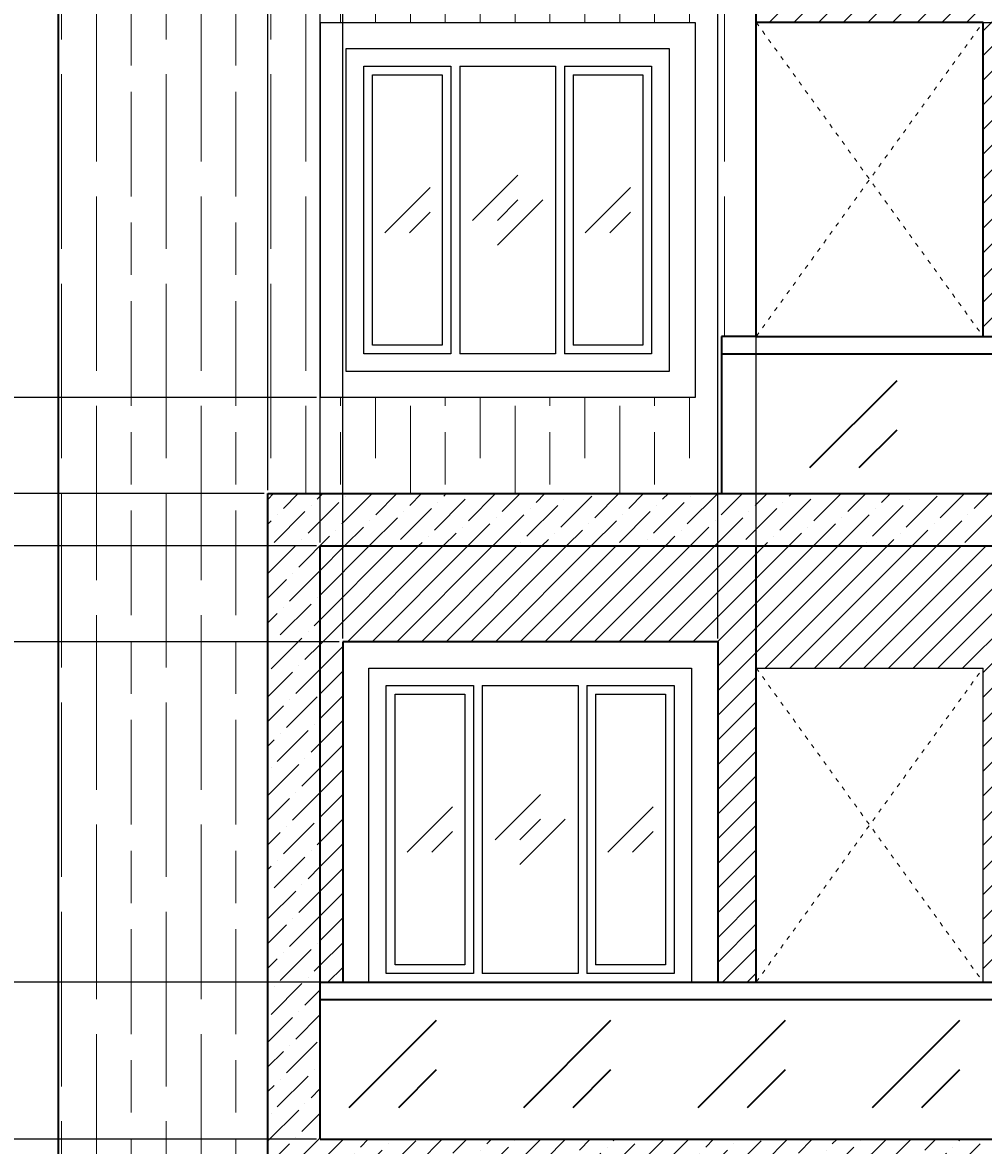
# Model space of a CAD drawing. Units: millimetres. Extents: x -692 to 9639, y -141 to 10345.
# Tile 13 of 19: x 3088 to 5843, y 4981 to 8199. Entities that reach past the tile are written whole.
import ezdxf

# ---------------------------------------------------------------- set-up
doc = ezdxf.new("R2010")
doc.units = ezdxf.units.MM
doc.header["$MEASUREMENT"] = 0
doc.linetypes.add('ACAD_ISO03W100', pattern=[30, 12, -18])
for name, color, linetype, lineweight in [('A-ANNO-DIMS', 2, 'Continuous', 18), ('A-DOOR', 3, 'Continuous', 25), ('A-DOOR-SWNG', 3, 'ACAD_ISO03W100', 18), ('A-ELEV', 7, 'Continuous', 35), ('A-ELEV-PATT', 8, 'Continuous', 13), ('A-GLAZ', 4, 'Continuous', 25)]:
    doc.layers.add(name, color=color, linetype=linetype, lineweight=lineweight)
doc.styles.get("Standard").update_dxf_attribs({"font": 'arial.ttf'})
doc.dimstyles.get("Standard").update_dxf_attribs({"dimtxt": 25, "dimasz": 20, "dimexe": 0.18, "dimexo": 10, "dimgap": 10, "dimtad": 0, "dimtih": 1, "dimtoh": 1, "dimdec": 0, "dimzin": 0, "dimdsep": 46, "dimtxsty": 'Standard', "dimcen": 10, "dimadec": 0, "dimazin": 0, "dimtfac": 1, "dimtdec": 0, "dimtofl": 0, "dimtmove": 0, "dimatfit": 3, "dimfxl": 1, "dimtolj": 1, "dimtzin": 0, "dimarcsym": 0})

# ---------------------------------------------------------------- blocks, each defined once
blk = doc.blocks.new('WIN-1075')
for p, q in [((0, 1075), (1075, 1075)), ((0, 1075), (0, 0)), ((1075, 1075), (1075, 0)), ((75, 1000), (1000, 1000)), ((75, 75), (75, 1000)), ((1000, 1000), (1000, 75)), ((125, 950), (375, 950)), ((125, 125), (125, 950)), ((375, 950), (375, 125)), ((400, 950), (400, 125)), ((400, 950), (675, 950)), ((675, 950), (675, 125)), ((700, 950), (700, 125)), ((700, 950), (950, 950)), ((950, 950), (950, 125)), ((150, 150), (150, 925)), ((150, 925), (350, 925)), ((350, 925), (350, 150)), ((725, 925), (725, 150)), ((725, 925), (925, 925)), ((925, 925), (925, 150)), ((567.1, 637.9), (437.1, 507.9)), ((315, 602.5), (185, 472.5)), ((890, 602.5), (760, 472.5)), ((637.9, 567.1), (507.9, 437.1)), ((567.1, 567.1), (507.9, 507.9)), ((315, 531.8), (255.7, 472.5)), ((890, 531.8), (830.7, 472.5)), ((350, 150), (150, 150)), ((925, 150), (725, 150)), ((375, 125), (125, 125)), ((675, 125), (400, 125)), ((950, 125), (700, 125)), ((1000, 75), (75, 75)), ((1075, 0), (0, 0))]:
    blk.add_line(p, q)
blk = doc.blocks.new('*D7')
at = {"layer": 'A-ANNO-DIMS', "color": 0, "lineweight": -2, "transparency": 16777216}
for p, q in [((8481.5, 9848.8), (-649.1, 9848.8)), ((-648.9, 9828.8), (-648.9, 5124.9)), ((-648.9, 375.6), (-648.9, 5079.4)), ((2463.7, 355.6), (-649.1, 355.6))]:
    blk.add_line(p, q, dxfattribs=at)
at = {"layer": 'A-ANNO-DIMS', "color": 0, "lineweight": -3, "transparency": 16777216}
for points in [[(-652.2, 9828.8), (-645.6, 9828.8), (-648.9, 9848.8)], [(-652.2, 375.6), (-645.6, 375.6), (-648.9, 355.6)]]:
    blk.add_solid(points, dxfattribs=at)
at = {"layer": 'Defpoints', "color": 0, "lineweight": -3, "transparency": 16777216}
for p in [(-648.9, 9848.8), (8491.5, 9848.8), (2473.7, 355.6)]:
    blk.add_point(p, dxfattribs=at)
at = {"layer": 'A-ANNO-DIMS', "color": 0, "transparency": 16777216, "insert": (-648.9, 5102.2), "char_height": 25, "attachment_point": 5}
blk.add_mtext('\\A1;9493', dxfattribs=at)
blk = doc.blocks.new('*D52')
at = {"layer": 'A-ANNO-DIMS', "color": 0, "lineweight": -2, "transparency": 16777216}
for p, q in [((3791.5, 6858.8), (3791.5, 10329)), ((3811.5, 10328.8), (3830.1, 10328.8)), ((3921.5, 10328.8), (3902.9, 10328.8)), ((3941.5, 6708.8), (3941.5, 10329))]:
    blk.add_line(p, q, dxfattribs=at)
at = {"layer": 'A-ANNO-DIMS', "color": 0, "lineweight": -3, "transparency": 16777216}
for points in [[(3811.5, 10332.1), (3811.5, 10325.4), (3791.5, 10328.8)], [(3921.5, 10332.1), (3921.5, 10325.4), (3941.5, 10328.8)]]:
    blk.add_solid(points, dxfattribs=at)
at = {"layer": 'Defpoints', "color": 0, "lineweight": -3, "transparency": 16777216}
for p in [(3941.5, 10328.8), (3791.5, 6848.8), (3941.5, 6698.8)]:
    blk.add_point(p, dxfattribs=at)
at = {"layer": 'A-ANNO-DIMS', "color": 0, "transparency": 16777216, "insert": (3866.5, 10328.8), "char_height": 25, "attachment_point": 5}
blk.add_mtext('\\A1;150', dxfattribs=at)
blk = doc.blocks.new('*D53')
at = {"layer": 'A-ANNO-DIMS', "color": 0, "lineweight": -2, "transparency": 16777216}
for p, q in [((3941.5, 6708.8), (3941.5, 10329)), ((3961.5, 10328.8), (3986.3, 10328.8)), ((4006.3, 6433.8), (4006.3, 10329)), ((4006.3, 10328.8), (4026.3, 10328.8))]:
    blk.add_line(p, q, dxfattribs=at)
at = {"layer": 'A-ANNO-DIMS', "color": 0, "lineweight": -3, "transparency": 16777216}
for points in [[(3961.5, 10332.1), (3961.5, 10325.4), (3941.5, 10328.8)], [(3986.3, 10332.1), (3986.3, 10325.4), (4006.3, 10328.8)]]:
    blk.add_solid(points, dxfattribs=at)
at = {"layer": 'Defpoints', "color": 0, "lineweight": -3, "transparency": 16777216}
for p in [(4006.3, 10328.8), (3941.5, 6698.8), (4006.3, 6423.8)]:
    blk.add_point(p, dxfattribs=at)
at = {"layer": 'A-ANNO-DIMS', "color": 0, "transparency": 16777216, "insert": (4076.1, 10328.8), "char_height": 25, "attachment_point": 5}
blk.add_mtext('\\A1;64.71', dxfattribs=at)
blk = doc.blocks.new('*D54')
at = {"layer": 'A-ANNO-DIMS', "color": 0, "lineweight": -2, "transparency": 16777216}
for p, q in [((4006.3, 6433.8), (4006.3, 10329)), ((4026.3, 10328.8), (4497.5, 10328.8)), ((5061.3, 10328.8), (4590, 10328.8)), ((5081.3, 6433.8), (5081.3, 10329))]:
    blk.add_line(p, q, dxfattribs=at)
at = {"layer": 'A-ANNO-DIMS', "color": 0, "lineweight": -3, "transparency": 16777216}
for points in [[(4026.3, 10332.1), (4026.3, 10325.4), (4006.3, 10328.8)], [(5061.3, 10332.1), (5061.3, 10325.4), (5081.3, 10328.8)]]:
    blk.add_solid(points, dxfattribs=at)
at = {"layer": 'Defpoints', "color": 0, "lineweight": -3, "transparency": 16777216}
for p in [(5081.3, 10328.8), (4006.3, 6423.8), (5081.3, 6423.8)]:
    blk.add_point(p, dxfattribs=at)
at = {"layer": 'A-ANNO-DIMS', "color": 0, "transparency": 16777216, "insert": (4543.8, 10328.8), "char_height": 25, "attachment_point": 5}
blk.add_mtext('\\A1;1075', dxfattribs=at)
blk = doc.blocks.new('*D55')
at = {"layer": 'A-ANNO-DIMS', "color": 0, "lineweight": -2, "transparency": 16777216}
for p, q in [((5081.3, 6433.8), (5081.3, 10329)), ((5101.3, 10328.8), (5171.5, 10328.8)), ((5191.5, 6358.8), (5191.5, 10329)), ((5191.5, 10328.8), (5211.5, 10328.8))]:
    blk.add_line(p, q, dxfattribs=at)
at = {"layer": 'A-ANNO-DIMS', "color": 0, "lineweight": -3, "transparency": 16777216}
for points in [[(5101.3, 10332.1), (5101.3, 10325.4), (5081.3, 10328.8)], [(5171.5, 10332.1), (5171.5, 10325.4), (5191.5, 10328.8)]]:
    blk.add_solid(points, dxfattribs=at)
at = {"layer": 'Defpoints', "color": 0, "lineweight": -3, "transparency": 16777216}
for p in [(5191.5, 10328.8), (5081.3, 6423.8), (5191.5, 6348.8)]:
    blk.add_point(p, dxfattribs=at)
at = {"layer": 'A-ANNO-DIMS', "color": 0, "transparency": 16777216, "insert": (5272.3, 10328.8), "char_height": 25, "attachment_point": 5}
blk.add_mtext('\\A1;110.29', dxfattribs=at)
blk = doc.blocks.new('*D56')
at = {"layer": 'A-ANNO-DIMS', "color": 0, "lineweight": -2, "transparency": 16777216}
for p, q in [((5191.5, 6358.8), (5191.5, 10329)), ((5211.5, 10328.8), (5981.1, 10328.8)), ((6871.7, 10328.8), (6102.2, 10328.8)), ((6891.7, 6708.8), (6891.7, 10329))]:
    blk.add_line(p, q, dxfattribs=at)
at = {"layer": 'A-ANNO-DIMS', "color": 0, "lineweight": -3, "transparency": 16777216}
for points in [[(5211.5, 10332.1), (5211.5, 10325.4), (5191.5, 10328.8)], [(6871.7, 10332.1), (6871.7, 10325.4), (6891.7, 10328.8)]]:
    blk.add_solid(points, dxfattribs=at)
at = {"layer": 'Defpoints', "color": 0, "lineweight": -3, "transparency": 16777216}
for p in [(6891.7, 10328.8), (6891.7, 6698.8), (5191.5, 6348.8)]:
    blk.add_point(p, dxfattribs=at)
at = {"layer": 'A-ANNO-DIMS', "color": 0, "transparency": 16777216, "insert": (6041.6, 10328.8), "char_height": 25, "attachment_point": 5}
blk.add_mtext('\\A1;1700.2', dxfattribs=at)
blk = doc.blocks.new('*D63')
at = {"layer": 'A-ANNO-DIMS', "color": 0, "lineweight": -2, "transparency": 16777216}
for p, q in [((3931.5, 4998.8), (-649.1, 4998.8)), ((-648.9, 4978.8), (-648.9, 4946.5)), ((-648.9, 4868.8), (-648.9, 4901)), ((3781.5, 4848.8), (-649.1, 4848.8))]:
    blk.add_line(p, q, dxfattribs=at)
at = {"layer": 'A-ANNO-DIMS', "color": 0, "lineweight": -3, "transparency": 16777216}
for points in [[(-652.2, 4978.8), (-645.6, 4978.8), (-648.9, 4998.8)], [(-652.2, 4868.8), (-645.6, 4868.8), (-648.9, 4848.8)]]:
    blk.add_solid(points, dxfattribs=at)
at = {"layer": 'Defpoints', "color": 0, "lineweight": -3, "transparency": 16777216}
for p in [(-648.9, 4998.8), (3941.5, 4998.8), (3791.5, 4848.8)]:
    blk.add_point(p, dxfattribs=at)
at = {"layer": 'A-ANNO-DIMS', "color": 0, "transparency": 16777216, "insert": (-648.9, 4923.8), "char_height": 25, "attachment_point": 5}
blk.add_mtext('\\A1;150', dxfattribs=at)
blk = doc.blocks.new('*D64')
at = {"layer": 'A-ANNO-DIMS', "color": 0, "lineweight": -2, "transparency": 16777216}
for p, q in [((3996.3, 5448.8), (-649.1, 5448.8)), ((-648.9, 5428.8), (-648.9, 5246.5)), ((-648.9, 5018.8), (-648.9, 5201)), ((3931.5, 4998.8), (-649.1, 4998.8))]:
    blk.add_line(p, q, dxfattribs=at)
at = {"layer": 'A-ANNO-DIMS', "color": 0, "lineweight": -3, "transparency": 16777216}
for points in [[(-652.2, 5428.8), (-645.6, 5428.8), (-648.9, 5448.8)], [(-652.2, 5018.8), (-645.6, 5018.8), (-648.9, 4998.8)]]:
    blk.add_solid(points, dxfattribs=at)
at = {"layer": 'Defpoints', "color": 0, "lineweight": -3, "transparency": 16777216}
for p in [(-648.9, 5448.8), (4006.3, 5448.8), (3941.5, 4998.8)]:
    blk.add_point(p, dxfattribs=at)
at = {"layer": 'A-ANNO-DIMS', "color": 0, "transparency": 16777216, "insert": (-648.9, 5223.8), "char_height": 25, "attachment_point": 5}
blk.add_mtext('\\A1;450', dxfattribs=at)
blk = doc.blocks.new('*D65')
at = {"layer": 'A-ANNO-DIMS', "color": 0, "lineweight": -2, "transparency": 16777216}
for p, q in [((3996.3, 6423.8), (-649.1, 6423.8)), ((-648.9, 6403.8), (-648.9, 5959)), ((-648.9, 5468.8), (-648.9, 5913.5)), ((3996.3, 5448.8), (-649.1, 5448.8))]:
    blk.add_line(p, q, dxfattribs=at)
at = {"layer": 'A-ANNO-DIMS', "color": 0, "lineweight": -3, "transparency": 16777216}
for points in [[(-652.2, 6403.8), (-645.6, 6403.8), (-648.9, 6423.8)], [(-652.2, 5468.8), (-645.6, 5468.8), (-648.9, 5448.8)]]:
    blk.add_solid(points, dxfattribs=at)
at = {"layer": 'Defpoints', "color": 0, "lineweight": -3, "transparency": 16777216}
for p in [(-648.9, 6423.8), (4006.3, 6423.8), (4006.3, 5448.8)]:
    blk.add_point(p, dxfattribs=at)
at = {"layer": 'A-ANNO-DIMS', "color": 0, "transparency": 16777216, "insert": (-648.9, 5936.3), "char_height": 25, "attachment_point": 5}
blk.add_mtext('\\A1;975', dxfattribs=at)
blk = doc.blocks.new('*D66')
at = {"layer": 'A-ANNO-DIMS', "color": 0, "lineweight": -2, "transparency": 16777216}
for p, q in [((3931.5, 6698.8), (-649.1, 6698.8)), ((-648.9, 6678.8), (-648.9, 6584)), ((-648.9, 6443.8), (-648.9, 6538.5)), ((3996.3, 6423.8), (-649.1, 6423.8))]:
    blk.add_line(p, q, dxfattribs=at)
at = {"layer": 'A-ANNO-DIMS', "color": 0, "lineweight": -3, "transparency": 16777216}
for points in [[(-652.2, 6678.8), (-645.6, 6678.8), (-648.9, 6698.8)], [(-652.2, 6443.8), (-645.6, 6443.8), (-648.9, 6423.8)]]:
    blk.add_solid(points, dxfattribs=at)
at = {"layer": 'Defpoints', "color": 0, "lineweight": -3, "transparency": 16777216}
for p in [(-648.9, 6698.8), (3941.5, 6698.8), (4006.3, 6423.8)]:
    blk.add_point(p, dxfattribs=at)
at = {"layer": 'A-ANNO-DIMS', "color": 0, "transparency": 16777216, "insert": (-648.9, 6561.3), "char_height": 25, "attachment_point": 5}
blk.add_mtext('\\A1;275', dxfattribs=at)
blk = doc.blocks.new('*D67')
at = {"layer": 'A-ANNO-DIMS', "color": 0, "lineweight": -2, "transparency": 16777216}
for p, q in [((3781.5, 6848.8), (-649.1, 6848.8)), ((-648.9, 6828.8), (-648.9, 6796.5)), ((-648.9, 6718.8), (-648.9, 6751)), ((3931.5, 6698.8), (-649.1, 6698.8))]:
    blk.add_line(p, q, dxfattribs=at)
at = {"layer": 'A-ANNO-DIMS', "color": 0, "lineweight": -3, "transparency": 16777216}
for points in [[(-652.2, 6828.8), (-645.6, 6828.8), (-648.9, 6848.8)], [(-652.2, 6718.8), (-645.6, 6718.8), (-648.9, 6698.8)]]:
    blk.add_solid(points, dxfattribs=at)
at = {"layer": 'Defpoints', "color": 0, "lineweight": -3, "transparency": 16777216}
for p in [(-648.9, 6848.8), (3791.5, 6848.8), (3941.5, 6698.8)]:
    blk.add_point(p, dxfattribs=at)
at = {"layer": 'A-ANNO-DIMS', "color": 0, "transparency": 16777216, "insert": (-648.9, 6773.8), "char_height": 25, "attachment_point": 5}
blk.add_mtext('\\A1;150', dxfattribs=at)
blk = doc.blocks.new('*D68')
at = {"layer": 'A-ANNO-DIMS', "color": 0, "lineweight": -2, "transparency": 16777216}
for p, q in [((3931.5, 7123.8), (-649.1, 7123.8)), ((-648.9, 7103.8), (-648.9, 7009)), ((-648.9, 6868.8), (-648.9, 6963.5)), ((3781.5, 6848.8), (-649.1, 6848.8))]:
    blk.add_line(p, q, dxfattribs=at)
at = {"layer": 'A-ANNO-DIMS', "color": 0, "lineweight": -3, "transparency": 16777216}
for points in [[(-652.2, 7103.8), (-645.6, 7103.8), (-648.9, 7123.8)], [(-652.2, 6868.8), (-645.6, 6868.8), (-648.9, 6848.8)]]:
    blk.add_solid(points, dxfattribs=at)
at = {"layer": 'Defpoints', "color": 0, "lineweight": -3, "transparency": 16777216}
for p in [(-648.9, 7123.8), (3941.5, 7123.8), (3791.5, 6848.8)]:
    blk.add_point(p, dxfattribs=at)
at = {"layer": 'A-ANNO-DIMS', "color": 0, "transparency": 16777216, "insert": (-648.9, 6986.3), "char_height": 25, "attachment_point": 5}
blk.add_mtext('\\A1;275', dxfattribs=at)
blk = doc.blocks.new('*D76')
at = {"layer": 'A-ANNO-DIMS', "color": 0, "lineweight": -2, "transparency": 16777216}
for p, q in [((5101.5, 7298.8), (9553.9, 7298.8)), ((9553.7, 7278.8), (9553.7, 7096.5)), ((9553.7, 6868.8), (9553.7, 7051)), ((5101.5, 6848.8), (9553.9, 6848.8))]:
    blk.add_line(p, q, dxfattribs=at)
at = {"layer": 'A-ANNO-DIMS', "color": 0, "lineweight": -3, "transparency": 16777216}
for points in [[(9550.4, 7278.8), (9557.1, 7278.8), (9553.7, 7298.8)], [(9550.4, 6868.8), (9557.1, 6868.8), (9553.7, 6848.8)]]:
    blk.add_solid(points, dxfattribs=at)
at = {"layer": 'Defpoints', "color": 0, "lineweight": -3, "transparency": 16777216}
for p in [(5091.5, 7298.8), (9553.7, 7298.8), (5091.5, 6848.8)]:
    blk.add_point(p, dxfattribs=at)
at = {"layer": 'A-ANNO-DIMS', "color": 0, "transparency": 16777216, "insert": (9553.7, 7073.8), "char_height": 25, "attachment_point": 5}
blk.add_mtext('\\A1;450', dxfattribs=at)
blk = doc.blocks.new('*D77')
at = {"layer": 'A-ANNO-DIMS', "color": 0, "lineweight": -2, "transparency": 16777216}
for p, q in [((5201.5, 8198.8), (9553.9, 8198.8)), ((9553.7, 8178.8), (9553.7, 7771.8)), ((9553.7, 7319.3), (9553.7, 7726.3)), ((5201.5, 7299.3), (9553.9, 7299.3))]:
    blk.add_line(p, q, dxfattribs=at)
at = {"layer": 'A-ANNO-DIMS', "color": 0, "lineweight": -3, "transparency": 16777216}
for points in [[(9550.4, 8178.8), (9557.1, 8178.8), (9553.7, 8198.8)], [(9550.4, 7319.3), (9557.1, 7319.3), (9553.7, 7299.3)]]:
    blk.add_solid(points, dxfattribs=at)
at = {"layer": 'Defpoints', "color": 0, "lineweight": -3, "transparency": 16777216}
for p in [(5191.5, 8198.8), (9553.7, 8198.8), (5191.5, 7299.3)]:
    blk.add_point(p, dxfattribs=at)
at = {"layer": 'A-ANNO-DIMS', "color": 0, "transparency": 16777216, "insert": (9553.7, 7749), "char_height": 25, "attachment_point": 5}
blk.add_mtext('\\A1;899.5', dxfattribs=at)

msp = doc.modelspace()

# ---------------------------------------------------------------- hatches: boundary and pattern name
at = {"layer": 'A-ELEV-PATT'}
h = msp.add_hatch(dxfattribs=at)
h.set_pattern_fill('GOST_WOOD', color=256, scale=50)
h.set_pattern_definition([(90, (0, 0), (300, -2e-14), [500, -100]), (90, (100, -100), (300, -2e-14), [300, -75, 150, -75]), (90, (200, -250), (300, -2e-14), [500, -100])])
edge = h.paths.add_edge_path()
edge.add_line((5191.547, 8748.772), (3791.547, 8748.772))
edge.add_line((3791.547, 8748.772), (3791.547, 8848.772))
edge.add_line((3791.547, 8848.772), (5191.547, 8848.772))
edge.add_line((5191.547, 8848.772), (5191.547, 9348.772))
edge.add_line((5191.547, 9348.772), (4755.992, 9348.772))
edge.add_line((4755.992, 9348.772), (4755.854, 9348.465))
edge.add_line((4755.854, 9348.465), (4755.734, 9348.772))
edge.add_line((4755.734, 9348.772), (4053.129, 9348.772))
edge.add_line((4053.129, 9348.772), (4052.99, 9348.465))
edge.add_line((4052.99, 9348.465), (4052.871, 9348.772))
edge.add_line((4052.871, 9348.772), (3701.731, 9348.772))
edge.add_line((3701.731, 9348.772), (3701.593, 9348.465))
edge.add_line((3701.593, 9348.465), (3701.474, 9348.772))
edge.add_line((3701.474, 9348.772), (3368.199, 9348.772))
edge.add_line((3368.199, 9348.772), (3368.061, 9348.465))
edge.add_line((3368.061, 9348.465), (3367.942, 9348.772))
edge.add_line((3367.942, 9348.772), (3191.547, 9348.772))
edge.add_line((3191.547, 9348.772), (3191.547, 3210.058))
edge.add_spline(control_points=[(3191.547, 3210.058), (3198.467, 3207.5), (3283.859, 3166.656), (3324.053, 2995.08), (3234.02, 2920.058), (3220.783, 2911.684)], knot_values=[13649.89756952, 13649.89756952, 13649.89756952, 13649.89756952, 13672.14990348, 13935.42377748, 13974.4426778, 13974.4426778, 13974.4426778, 13974.4426778], degree=3, periodic=0)
edge.add_spline(control_points=[(3220.783, 2911.684), (3225.148, 2890.107), (3226.864, 2868.931), (3226.144, 2848.27)], knot_values=[8828.69997321, 8828.69997321, 8828.69997321, 8828.69997321, 8890.6429847, 8890.6429847, 8890.6429847, 8890.6429847], degree=3, periodic=0)
edge.add_line((3226.144, 2848.27), (5191.547, 2848.27))
edge.add_line((5191.547, 2848.27), (5191.547, 3048.27))
edge.add_line((5191.547, 3048.27), (5041.547, 3048.27))
edge.add_line((5041.547, 3048.27), (5041.547, 3148.27))
edge.add_line((5041.547, 3148.27), (5091.547, 3148.27))
edge.add_line((5091.547, 3148.27), (5091.547, 3598.27))
edge.add_line((5091.547, 3598.27), (5191.547, 3598.27))
edge.add_line((5191.547, 3598.27), (5191.547, 4848.772))
edge.add_line((5191.547, 4848.772), (3791.547, 4848.772))
edge.add_line((3791.547, 4848.772), (3791.547, 6848.772))
edge.add_line((3791.547, 6848.772), (5091.547, 6848.772))
edge.add_line((5091.547, 6848.772), (5091.547, 7298.772))
edge.add_line((5091.547, 7298.772), (5191.547, 7298.772))
edge.add_line((5191.547, 7298.772), (5191.547, 8748.772))
h.paths.add_polyline_path([(5016.547, 8198.772), (5016.547, 7123.772), (3941.547, 7123.772), (3941.547, 8198.772)], flags=16)
h.paths.add_polyline_path([(4941.547, 8123.772), (4941.547, 7198.772), (4016.547, 7198.772), (4016.547, 8123.772)], flags=0)
h.paths.add_polyline_path([(4616.547, 8073.772), (4616.547, 7248.772), (4341.547, 7248.772), (4341.547, 8073.772)], flags=0)
h.paths.add_polyline_path([(4641.547, 8073.772), (4891.547, 8073.772), (4891.547, 7248.772), (4641.547, 7248.772)], flags=0)
h.paths.add_polyline_path([(4666.547, 8048.772), (4866.547, 8048.772), (4866.547, 7273.772), (4666.547, 7273.772)], flags=0)
h.paths.add_polyline_path([(4316.547, 8073.772), (4316.547, 7248.772), (4066.547, 7248.772), (4066.547, 8073.772)], flags=0)
h.paths.add_polyline_path([(4291.547, 8048.772), (4291.547, 7273.772), (4091.547, 7273.772), (4091.547, 8048.772)], flags=0)
h.paths.add_polyline_path([(5016.547, 4497.772), (5016.547, 3422.772), (3941.547, 3422.772), (3941.547, 4497.772)], flags=16)
h.paths.add_polyline_path([(4941.547, 4422.772), (4941.547, 3497.772), (4016.547, 3497.772), (4016.547, 4422.772)], flags=0)
h.paths.add_polyline_path([(4616.547, 4372.772), (4616.547, 3547.772), (4341.547, 3547.772), (4341.547, 4372.772)], flags=0)
h.paths.add_polyline_path([(4641.547, 4372.772), (4891.547, 4372.772), (4891.547, 3547.772), (4641.547, 3547.772)], flags=0)
h.paths.add_polyline_path([(4316.547, 4372.772), (4316.547, 3547.772), (4066.547, 3547.772), (4066.547, 4372.772)], flags=0)
h.paths.add_polyline_path([(4666.547, 4347.772), (4866.547, 4347.772), (4866.547, 3572.772), (4666.547, 3572.772)], flags=0)
h.paths.add_polyline_path([(4291.547, 4347.772), (4291.547, 3572.772), (4091.547, 3572.772), (4091.547, 4347.772)], flags=0)
h = msp.add_hatch(dxfattribs=at)
h.set_pattern_fill('ANSI31', color=256, scale=400)
h.paths.add_polyline_path([(6891.746, 6698.772), (5191.547, 6698.772), (5191.547, 6348.772), (5841.547, 6348.772), (5841.547, 5448.772), (6041.547, 5448.772), (6041.547, 6348.772), (6691.547, 6348.772), (6691.547, 5448.772), (6891.746, 5448.772)])
h.paths.add_polyline_path([(5191.547, 6698.772), (3941.547, 6698.772), (3941.547, 5448.772), (4006.259, 5448.772), (4006.259, 6423.772), (5081.259, 6423.772), (5081.259, 5448.772), (5191.547, 5448.772), (5191.547, 6348.772)])
h.paths.add_polyline_path([(6891.746, 4848.772), (5191.547, 4848.772), (5191.547, 4497.772), (5841.746, 4497.772), (5841.746, 3598.27), (6041.746, 3598.27), (6041.746, 4497.772), (6691.746, 4497.772), (6691.746, 3598.27), (6891.746, 3598.27)])
h.paths.add_polyline_path([(6891.746, 8748.772), (5191.547, 8748.772), (5191.547, 8198.772), (5841.547, 8198.772), (5841.547, 7298.772), (6041.547, 7298.772), (6041.547, 8198.772), (6691.547, 8198.772), (6691.547, 7298.772), (6891.746, 7298.772)])
h = msp.add_hatch(dxfattribs=at)
h.set_pattern_fill('ANSI36', color=256, scale=400)
h.paths.add_polyline_path([(8691.547, 6848.772), (3791.547, 6848.772), (3791.547, 4848.772), (8691.547, 4848.772), (8691.547, 4998.772), (3941.547, 4998.772), (3941.547, 6698.772), (8691.547, 6698.772)])

# ---------------------------------------------------------------- linework, layer by layer
at = {"layer": 'A-DOOR'}
for p, q in [((5191.547, 5448.772), (5191.547, 6348.772)), ((5191.547, 6348.772), (5841.547, 6348.772)), ((5841.547, 5448.772), (5841.547, 6348.772))]:
    msp.add_line(p, q, dxfattribs=at)
at = {"layer": 'A-DOOR-SWNG'}
for p, q in [((5191.547, 7299.27), (5841.746, 8198.772)), ((5191.547, 8198.772), (5841.746, 7299.27)), ((5191.547, 5449.27), (5841.746, 6348.772)), ((5191.547, 6348.772), (5841.746, 5449.27))]:
    msp.add_line(p, q, dxfattribs=at)
at = {"layer": 'A-ELEV'}
for p, q in [((3191.547, 2848.27), (3191.547, 9348.772)), ((5191.547, 7298.772), (5191.547, 8748.772)), ((5841.547, 8198.772), (5191.547, 8198.772)), ((5841.547, 7298.772), (5841.547, 8198.772)), ((5191.547, 7298.772), (5091.547, 7298.772)), ((5091.547, 7298.772), (5091.547, 6848.772)), ((5191.547, 7298.772), (8391.547, 7298.772)), ((5091.547, 7248.772), (8391.547, 7248.772)), ((5594.403, 7172.266), (5344.403, 6922.266)), ((5594.403, 7030.844), (5485.824, 6922.266)), ((3791.547, 6848.772), (8691.547, 6848.772)), ((3791.547, 4848.772), (3791.547, 6848.772)), ((3941.547, 6698.772), (8691.547, 6698.772)), ((3941.547, 4998.772), (3941.547, 6698.772)), ((5191.547, 5448.772), (5191.547, 6698.772)), ((4006.259, 6423.772), (4006.259, 5448.772)), ((5081.259, 6423.772), (4006.259, 6423.772)), ((5081.259, 6423.772), (5081.259, 5448.772)), ((3941.547, 5448.772), (6891.746, 5448.772)), ((3941.547, 5398.772), (6891.746, 5398.772)), ((4274.259, 5338.983), (4024.259, 5088.983)), ((4774.259, 5338.983), (4524.259, 5088.983)), ((5274.259, 5338.983), (5024.259, 5088.983)), ((5774.259, 5338.983), (5524.259, 5088.983)), ((4274.259, 5197.562), (4165.681, 5088.983)), ((4774.259, 5197.562), (4665.681, 5088.983)), ((5274.259, 5197.562), (5165.681, 5088.983)), ((5774.259, 5197.562), (5665.681, 5088.983)), ((3941.547, 4998.772), (8691.547, 4998.772))]:
    msp.add_line(p, q, dxfattribs=at)
at = {"layer": 'A-GLAZ'}
for p, q in [((4081.259, 6348.772), (5006.259, 6348.772)), ((4081.259, 5448.772), (4081.259, 6348.772)), ((5006.259, 6348.772), (5006.259, 5448.772)), ((4131.259, 6298.772), (4381.259, 6298.772)), ((4131.259, 5473.772), (4131.259, 6298.772)), ((4381.259, 6298.772), (4381.259, 5473.772)), ((4406.259, 6298.772), (4681.259, 6298.772)), ((4406.259, 6298.772), (4406.259, 5473.772)), ((4681.259, 6298.772), (4681.259, 5473.772)), ((4706.259, 6298.772), (4956.259, 6298.772)), ((4706.259, 6298.772), (4706.259, 5473.772)), ((4956.259, 6298.772), (4956.259, 5473.772)), ((4156.259, 6273.772), (4356.259, 6273.772)), ((4156.259, 5498.772), (4156.259, 6273.772)), ((4356.259, 6273.772), (4356.259, 5498.772)), ((4731.259, 6273.772), (4931.259, 6273.772)), ((4731.259, 6273.772), (4731.259, 5498.772)), ((4931.259, 6273.772), (4931.259, 5498.772)), ((4573.403, 5986.627), (4443.403, 5856.627)), ((4321.259, 5951.272), (4191.259, 5821.272)), ((4896.259, 5951.272), (4766.259, 5821.272)), ((4644.114, 5915.917), (4514.114, 5785.917)), ((4573.403, 5915.917), (4514.114, 5856.627)), ((4321.259, 5880.561), (4261.969, 5821.272)), ((4896.259, 5880.561), (4836.969, 5821.272)), ((4381.259, 5473.772), (4131.259, 5473.772)), ((4356.259, 5498.772), (4156.259, 5498.772)), ((4681.259, 5473.772), (4406.259, 5473.772)), ((4956.259, 5473.772), (4706.259, 5473.772)), ((4931.259, 5498.772), (4731.259, 5498.772))]:
    msp.add_line(p, q, dxfattribs=at)

# ---------------------------------------------------------------- block references
msp.add_blockref('WIN-1075', (3941.547, 7123.772), dxfattribs=at)

# ---------------------------------------------------------------- dimensions: what is measured, and where the dimension line sits
at = {"layer": 'A-ANNO-DIMS'}
for base, p1, p2, override, picture, middle in [((3941.547, 10328.772), (3791.547, 6848.772), (3941.547, 6698.772), {"dimdec": 0, "dimlfac": 1, "dimrnd": 0, "dimzin": 0, "dimdsep": 46, "dimlunit": 2}, '*D52', (3866.547, 10328.772)), ((4006.259, 10328.772), (3941.547, 6698.772), (4006.259, 6423.772), {"dimdec": 2, "dimlfac": 1, "dimrnd": 0, "dimzin": 0, "dimdsep": 46, "dimlunit": 2}, '*D53', (4076.095, 10328.772)), ((5081.259, 10328.772), (4006.259, 6423.772), (5081.259, 6423.772), {"dimdec": 0, "dimlfac": 1, "dimrnd": 0, "dimzin": 0, "dimdsep": 46, "dimlunit": 2}, '*D54', (4543.759, 10328.772)), ((5191.547, 10328.772), (5081.259, 6423.772), (5191.547, 6348.772), {"dimdec": 2, "dimlfac": 1, "dimrnd": 0, "dimzin": 0, "dimdsep": 46, "dimlunit": 2}, '*D55', (5272.288, 10328.772)), ((6891.746, 10328.772), (5191.547, 6348.772), (6891.746, 6698.772), {"dimdec": 1, "dimlfac": 1, "dimrnd": 0, "dimzin": 0, "dimdsep": 46, "dimlunit": 2}, '*D56', (6041.646, 10328.772))]:
    dim = msp.add_linear_dim(base=base, p1=p1, p2=p2, dimstyle='Standard', override=override, dxfattribs=at)
    dim.commit()
    dim.dimension.update_dxf_attribs({"geometry": picture, "text_midpoint": middle})
for base, p1, p2, override, picture, middle in [((-648.912, 9848.772), (2473.746, 355.575), (8491.547, 9848.772), {"dimdec": 0, "dimlfac": 1, "dimrnd": 0, "dimzin": 0, "dimdsep": 46, "dimlunit": 2}, '*D7', (-648.912, 5102.173)), ((9553.746, 8198.772), (5191.547, 7299.27), (5191.547, 8198.772), {"dimdec": 1, "dimlfac": 1, "dimrnd": 0, "dimzin": 0, "dimdsep": 46, "dimlunit": 2}, '*D77', (9553.746, 7749.021)), ((9553.746, 7298.772), (5091.547, 6848.772), (5091.547, 7298.772), {"dimdec": 0, "dimlfac": 1, "dimrnd": 0, "dimzin": 0, "dimdsep": 46, "dimlunit": 2}, '*D76', (9553.746, 7073.772)), ((-648.912, 7123.772), (3791.547, 6848.772), (3941.547, 7123.772), {"dimdec": 0, "dimlfac": 1, "dimrnd": 0, "dimzin": 0, "dimdsep": 46, "dimlunit": 2}, '*D68', (-648.912, 6986.272)), ((-648.912, 6848.772), (3941.547, 6698.772), (3791.547, 6848.772), {"dimdec": 0, "dimlfac": 1, "dimrnd": 0, "dimzin": 0, "dimdsep": 46, "dimlunit": 2}, '*D67', (-648.912, 6773.772)), ((-648.912, 6698.772), (4006.259, 6423.772), (3941.547, 6698.772), {"dimdec": 0, "dimlfac": 1, "dimrnd": 0, "dimzin": 0, "dimdsep": 46, "dimlunit": 2}, '*D66', (-648.912, 6561.272)), ((-648.912, 6423.772), (4006.259, 5448.772), (4006.259, 6423.772), {"dimdec": 0, "dimlfac": 1, "dimrnd": 0, "dimzin": 0, "dimdsep": 46, "dimlunit": 2}, '*D65', (-648.912, 5936.272)), ((-648.912, 5448.772), (3941.547, 4998.772), (4006.259, 5448.772), {"dimdec": 0, "dimlfac": 1, "dimrnd": 0, "dimzin": 0, "dimdsep": 46, "dimlunit": 2}, '*D64', (-648.912, 5223.772)), ((-648.912, 4998.772), (3791.547, 4848.772), (3941.547, 4998.772), {"dimdec": 0, "dimlfac": 1, "dimrnd": 0, "dimzin": 0, "dimdsep": 46, "dimlunit": 2}, '*D63', (-648.912, 4923.772))]:
    dim = msp.add_linear_dim(base=base, p1=p1, p2=p2, angle=90, dimstyle='Standard', override=override, dxfattribs=at)
    dim.commit()
    dim.dimension.update_dxf_attribs({"geometry": picture, "text_midpoint": middle})

doc.saveas('drawing.dxf')
